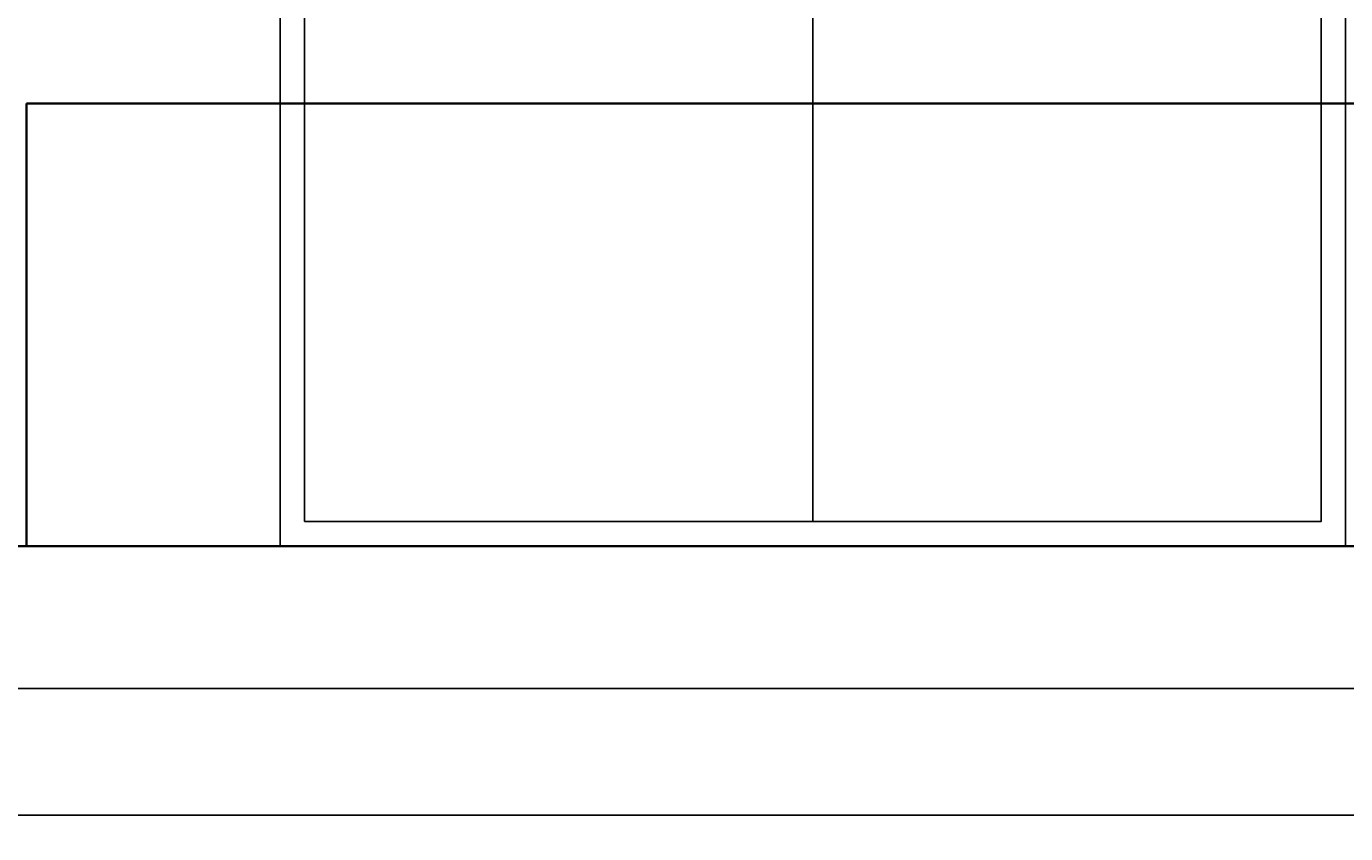
# Model space of a CAD drawing. Units: inches. Extents: x -145 to 510, y 5 to 386.
# Tile 11 of 25: x 75 to 182, y 177 to 242. Entities that reach past the tile are written whole.
import ezdxf

# ---------------------------------------------------------------- set-up
doc = ezdxf.new("R2010")
doc.units = ezdxf.units.IN
doc.header["$MEASUREMENT"] = 0
for name, color, linetype, lineweight in [('A-ANNO-DIMS', 2, 'Continuous', 18), ('A-ELEV', 7, 'Continuous', 35), ('A-GLAZ', 4, 'Continuous', 25)]:
    doc.layers.add(name, color=color, linetype=linetype, lineweight=lineweight)
doc.styles.get("Standard").update_dxf_attribs({"font": 'arial.ttf'})
doc.dimstyles.get("Standard").update_dxf_attribs({"dimtxt": 0.6875, "dimasz": 0.18, "dimexe": 0.18, "dimexo": 0.0625, "dimgap": 0.09, "dimtad": 0, "dimtih": 1, "dimtoh": 1, "dimdec": 4, "dimzin": 0, "dimdsep": 46, "dimlunit": 4, "dimtxsty": 'Standard', "dimcen": 0.09, "dimadec": 0, "dimazin": 0, "dimtfac": 1, "dimtdec": 4, "dimtofl": 0, "dimtmove": 0, "dimatfit": 3, "dimfxl": 1, "dimtolj": 1, "dimtzin": 0, "dimarcsym": 0})

# ---------------------------------------------------------------- blocks, each defined once
blk = doc.blocks.new('*D15')
at = {"layer": 'A-ANNO-DIMS', "color": 0, "lineweight": -2, "transparency": 16777216}
for p, q in [((69.78, 199.95), (69.78, 385.97)), ((69.96, 385.79), (80.93, 385.79)), ((94.96, 385.79), (83.98, 385.79)), ((95.14, 305.8), (95.14, 385.97))]:
    blk.add_line(p, q, dxfattribs=at)
at = {"layer": 'A-ANNO-DIMS', "color": 0, "transparency": 16777216}
for points in [[(69.96, 385.82), (69.96, 385.76), (69.78, 385.79)], [(94.96, 385.82), (94.96, 385.76), (95.14, 385.79)]]:
    blk.add_solid(points, dxfattribs=at)
at = {"layer": 'Defpoints', "color": 0, "transparency": 16777216}
for p in [(95.14, 385.79), (95.14, 305.74), (69.78, 199.89)]:
    blk.add_point(p, dxfattribs=at)
at = {"layer": 'A-ANNO-DIMS', "color": 0, "transparency": 16777216, "insert": (82.46, 385.79), "char_height": 0.688, "attachment_point": 5}
blk.add_mtext('\\A1;25.365', dxfattribs=at)
blk = doc.blocks.new('*D19')
at = {"layer": 'A-ANNO-DIMS', "color": 0, "lineweight": -2, "transparency": 16777216}
for p, q in [((478.76, 355.89), (-144.05, 355.89)), ((-143.87, 355.71), (-143.87, 218.33)), ((-143.87, 80.07), (-143.87, 217.45)), ((-114.04, 79.89), (-144.05, 79.89))]:
    blk.add_line(p, q, dxfattribs=at)
at = {"layer": 'A-ANNO-DIMS', "color": 0, "transparency": 16777216}
for points in [[(-143.9, 355.71), (-143.84, 355.71), (-143.87, 355.89)], [(-143.9, 80.07), (-143.84, 80.07), (-143.87, 79.89)]]:
    blk.add_solid(points, dxfattribs=at)
at = {"layer": 'Defpoints', "color": 0, "transparency": 16777216}
for p in [(-143.87, 355.89), (478.83, 355.89), (-113.97, 79.89)]:
    blk.add_point(p, dxfattribs=at)
at = {"layer": 'A-ANNO-DIMS', "color": 0, "transparency": 16777216, "insert": (-143.87, 217.89), "char_height": 0.688, "attachment_point": 5}
blk.add_mtext('\\A1;276', dxfattribs=at)
blk = doc.blocks.new('*D26')
at = {"layer": 'A-ANNO-DIMS', "color": 0, "lineweight": -2, "transparency": 16777216}
for p, q in [((95.08, 305.74), (-144.05, 305.74)), ((-143.87, 305.56), (-143.87, 253.26)), ((-143.87, 200.07), (-143.87, 252.38)), ((95.08, 199.89), (-144.05, 199.89))]:
    blk.add_line(p, q, dxfattribs=at)
at = {"layer": 'A-ANNO-DIMS', "color": 0, "transparency": 16777216}
for points in [[(-143.9, 305.56), (-143.84, 305.56), (-143.87, 305.74)], [(-143.9, 200.07), (-143.84, 200.07), (-143.87, 199.89)]]:
    blk.add_solid(points, dxfattribs=at)
at = {"layer": 'Defpoints', "color": 0, "transparency": 16777216}
for p in [(-143.87, 305.74), (95.14, 305.74), (95.14, 199.89)]:
    blk.add_point(p, dxfattribs=at)
at = {"layer": 'A-ANNO-DIMS', "color": 0, "transparency": 16777216, "insert": (-143.87, 252.82), "char_height": 0.688, "attachment_point": 5}
blk.add_mtext('\\A1;105.85', dxfattribs=at)
blk = doc.blocks.new('*D27')
at = {"layer": 'A-ANNO-DIMS', "color": 0, "lineweight": -2, "transparency": 16777216}
for p, q in [((244.23, 279.84), (-144.05, 279.84)), ((-143.87, 279.66), (-143.87, 240.31)), ((-143.87, 200.07), (-143.87, 239.43)), ((218.29, 199.89), (-144.05, 199.89))]:
    blk.add_line(p, q, dxfattribs=at)
at = {"layer": 'A-ANNO-DIMS', "color": 0, "transparency": 16777216}
for points in [[(-143.9, 279.66), (-143.84, 279.66), (-143.87, 279.84)], [(-143.9, 200.07), (-143.84, 200.07), (-143.87, 199.89)]]:
    blk.add_solid(points, dxfattribs=at)
at = {"layer": 'Defpoints', "color": 0, "transparency": 16777216}
for p in [(-143.87, 279.84), (244.29, 279.84), (218.36, 199.89)]:
    blk.add_point(p, dxfattribs=at)
at = {"layer": 'A-ANNO-DIMS', "color": 0, "transparency": 16777216, "insert": (-143.87, 239.87), "char_height": 0.688, "attachment_point": 5}
blk.add_mtext('\\A1;79.95', dxfattribs=at)
blk = doc.blocks.new('*D30')
at = {"layer": 'A-ANNO-DIMS', "color": 0, "lineweight": -2, "transparency": 16777216}
for p, q in [((210.73, 188.31), (-144.05, 188.31)), ((-143.87, 188.13), (-143.87, 183.61)), ((-143.87, 178.2), (-143.87, 182.72)), ((210.73, 178.02), (-144.05, 178.02))]:
    blk.add_line(p, q, dxfattribs=at)
at = {"layer": 'A-ANNO-DIMS', "color": 0, "transparency": 16777216}
for points in [[(-143.9, 188.13), (-143.84, 188.13), (-143.87, 188.31)], [(-143.9, 178.2), (-143.84, 178.2), (-143.87, 178.02)]]:
    blk.add_solid(points, dxfattribs=at)
at = {"layer": 'Defpoints', "color": 0, "transparency": 16777216}
for p in [(-143.87, 188.31), (210.8, 188.31), (210.8, 178.02)]:
    blk.add_point(p, dxfattribs=at)
at = {"layer": 'A-ANNO-DIMS', "color": 0, "transparency": 16777216, "insert": (-143.87, 183.16), "char_height": 0.688, "attachment_point": 5}
blk.add_mtext('\\A1;10.29', dxfattribs=at)

msp = doc.modelspace()

# ---------------------------------------------------------------- linework, layer by layer
at = {"layer": 'A-ELEV'}
for p, q in [((74.5073, 199.8905), (74.5073, 235.8905)), ((74.5073, 235.8905), (212.8652, 235.8905)), ((218.3571, 199.8905), (54.0014, 199.8905))]:
    msp.add_line(p, q, dxfattribs=at)
at = {"layer": 'A-GLAZ'}
msp.add_line((138.4805, 303.7416), (138.4805, 201.8905), dxfattribs=at)
for points in [[(95.1414, 199.8905), (181.8195, 199.8905), (181.8195, 305.7416), (95.1414, 305.7416)], [(97.1414, 201.8905), (179.8195, 201.8905), (179.8195, 303.7416), (97.1414, 303.7416)]]:
    msp.add_lwpolyline(points, close=True, dxfattribs=at)

# ---------------------------------------------------------------- dimensions: what is measured, and where the dimension line sits
at = {"layer": 'A-ANNO-DIMS'}
dim = msp.add_linear_dim(base=(95.1414, 385.7905), p1=(69.7763, 199.8905), p2=(95.1414, 305.7416), dimstyle='Standard', override={"dimdec": 3, "dimlfac": 1, "dimrnd": 0, "dimzin": 0, "dimdsep": 46, "dimlunit": 2}, dxfattribs=at)
dim.commit()
dim.dimension.update_dxf_attribs({"geometry": '*D15', "text_midpoint": (82.4589, 385.7905)})
for base, p1, p2, override, picture, middle in [((-143.8737, 355.8905), (-113.9737, 79.8905), (478.8263, 355.8905), {"dimdec": 0, "dimlfac": 1, "dimrnd": 0, "dimzin": 0, "dimdsep": 46, "dimlunit": 2}, '*D19', (-143.8737, 217.8905)), ((-143.8737, 305.7416), (95.1414, 199.8905), (95.1414, 305.7416), {"dimdec": 2, "dimlfac": 1, "dimrnd": 0, "dimzin": 0, "dimdsep": 46, "dimlunit": 2}, '*D26', (-143.8737, 252.8161)), ((-143.8737, 279.8443), (218.3571, 199.8905), (244.2916, 279.8443), {"dimdec": 2, "dimlfac": 1, "dimrnd": 0, "dimzin": 0, "dimdsep": 46, "dimlunit": 2}, '*D27', (-143.8737, 239.8674)), ((-143.8737, 188.3087), (210.7973, 178.0195), (210.7973, 188.3087), {"dimdec": 2, "dimlfac": 1, "dimrnd": 0, "dimzin": 0, "dimdsep": 46, "dimlunit": 2}, '*D30', (-143.8737, 183.1641))]:
    dim = msp.add_linear_dim(base=base, p1=p1, p2=p2, angle=90, dimstyle='Standard', override=override, dxfattribs=at)
    dim.commit()
    dim.dimension.update_dxf_attribs({"geometry": picture, "text_midpoint": middle})

doc.saveas('drawing.dxf')
